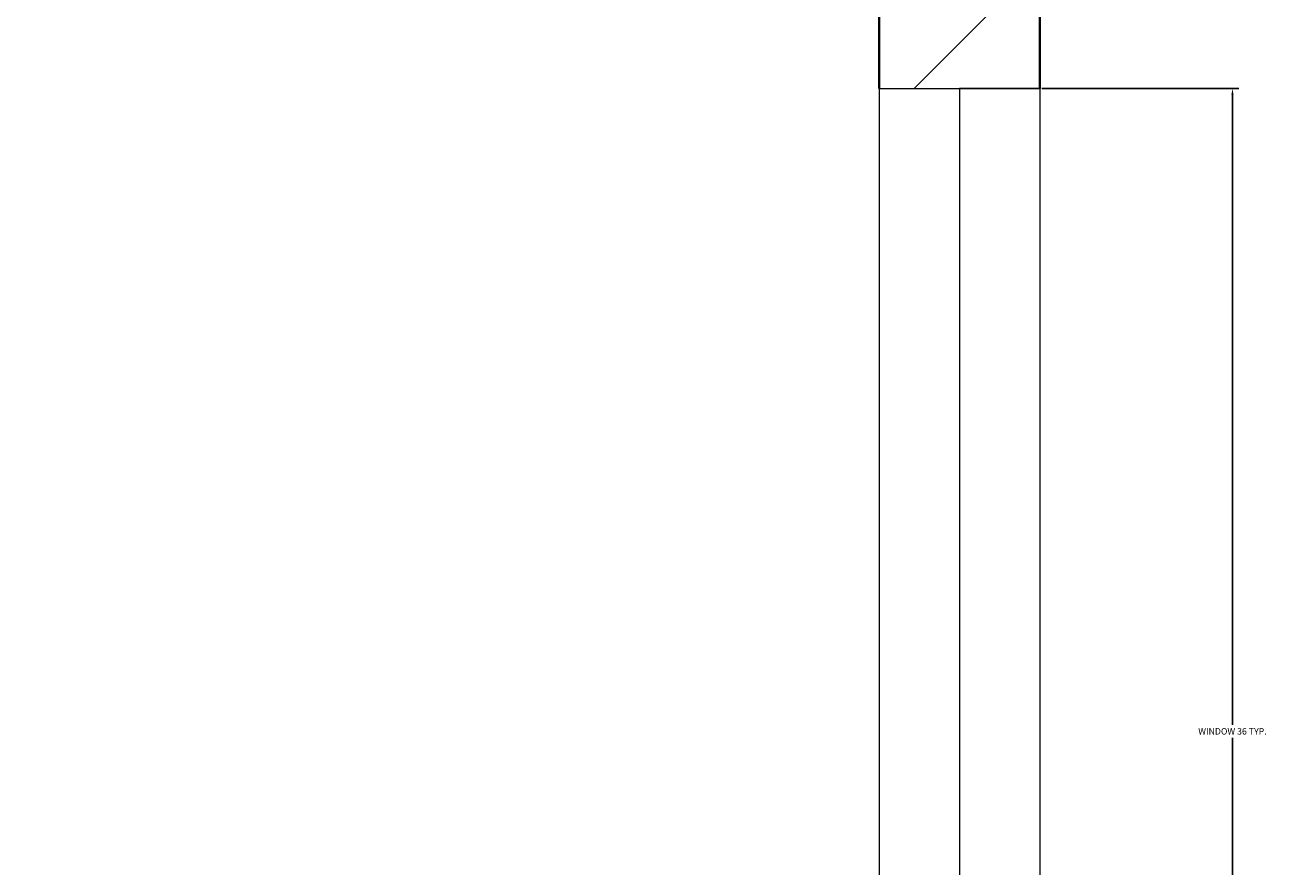
# Model space of a CAD drawing. Units: inches. Extents: x 1885 to 2748, y 783 to 2421.
# Tile 75 of 117: x 1969 to 2004, y 2120 to 2144. Entities that reach past the tile are written whole.
import ezdxf

# ---------------------------------------------------------------- set-up
doc = ezdxf.new("R2010")
doc.units = ezdxf.units.IN
for name, color, linetype, lineweight in [('A-ANNO-DIMS', 2, 'Continuous', 18), ('A-GLAZ', 181, 'Continuous', 18), ('A-WALL', 7, 'Continuous', 35)]:
    doc.layers.add(name, color=color, linetype=linetype, lineweight=lineweight)
doc.layers.add('A-WALL-PATT', color=85, linetype='Continuous', lineweight=13, true_color=0x58ba48)
doc.styles.get("Standard").update_dxf_attribs({"font": 'arial.ttf'})
doc.dimstyles.get("Standard").update_dxf_attribs({"dimtxt": 0.18, "dimasz": 0.18, "dimexe": 0.18, "dimexo": 0.0625, "dimgap": 0.09, "dimtad": 0, "dimtih": 1, "dimtoh": 1, "dimdec": 4, "dimzin": 0, "dimdsep": 46, "dimtxsty": 'Standard', "dimcen": 0.09, "dimadec": 0, "dimazin": 0, "dimtfac": 1, "dimtdec": 4, "dimtofl": 0, "dimtmove": 0, "dimatfit": 3, "dimfxl": 1, "dimtolj": 1, "dimtzin": 0, "dimarcsym": 0})

# ---------------------------------------------------------------- blocks, each defined once
blk = doc.blocks.new('WIN-36')
for p, q in [((0.004, 35.998), (4.504, 35.998)), ((0.004, 35.998), (0.004, -0.002)), ((4.504, 35.998), (2.254, 35.998)), ((2.254, 35.998), (2.254, -0.002)), ((4.504, 35.998), (4.504, -0.002)), ((2.254, -0.002), (0.004, -0.002)), ((0.004, -0.002), (4.504, -0.002))]:
    blk.add_line(p, q)
blk = doc.blocks.new('*D19')
at = {"layer": 'A-ANNO-DIMS', "color": 0, "lineweight": -2, "transparency": 16777216}
for p, q in [((1997.336, 2141.927), (2002.854, 2141.927)), ((2002.674, 2141.747), (2002.674, 2124.11)), ((2002.674, 2106.107), (2002.674, 2123.744)), ((1997.336, 2105.927), (2002.854, 2105.927))]:
    blk.add_line(p, q, dxfattribs=at)
at = {"layer": 'A-ANNO-DIMS', "color": 0, "transparency": 16777216}
for points in [[(2002.644, 2141.747), (2002.704, 2141.747), (2002.674, 2141.927)], [(2002.644, 2106.107), (2002.704, 2106.107), (2002.674, 2105.927)]]:
    blk.add_solid(points, dxfattribs=at)
at = {"layer": 'Defpoints', "color": 0, "transparency": 16777216}
for p in [(1997.274, 2141.927), (2002.674, 2141.927), (1997.274, 2105.927)]:
    blk.add_point(p, dxfattribs=at)
at = {"layer": 'A-ANNO-DIMS', "color": 0, "transparency": 16777216, "insert": (2002.674, 2123.927), "char_height": 0.18, "attachment_point": 5}
blk.add_mtext('\\A1;WINDOW 36 TYP.', dxfattribs=at)
blk = doc.blocks.new('*D48')
at = {"layer": 'A-ANNO-DIMS', "color": 0, "lineweight": -2, "transparency": 16777216}
for p, q in [((1980.711, 2348.006), (1902.844, 2348.006)), ((1903.024, 2347.826), (1903.024, 2114.937)), ((1903.024, 1881.686), (1903.024, 2114.574)), ((2016.711, 1881.506), (1902.844, 1881.506))]:
    blk.add_line(p, q, dxfattribs=at)
at = {"layer": 'A-ANNO-DIMS', "color": 0, "transparency": 16777216}
for points in [[(1902.994, 2347.826), (1903.054, 2347.826), (1903.024, 2348.006)], [(1902.994, 1881.686), (1903.054, 1881.686), (1903.024, 1881.506)]]:
    blk.add_solid(points, dxfattribs=at)
at = {"layer": 'Defpoints', "color": 0, "transparency": 16777216}
for p in [(1903.024, 2348.006), (1980.774, 2348.006), (2016.774, 1881.506)]:
    blk.add_point(p, dxfattribs=at)
at = {"layer": 'A-ANNO-DIMS', "color": 0, "transparency": 16777216, "insert": (1903.024, 2114.756), "char_height": 0.18, "attachment_point": 5}
blk.add_mtext('\\A1;466.5', dxfattribs=at)

msp = doc.modelspace()

# ---------------------------------------------------------------- hatches: boundary and pattern name
at = {"layer": 'A-WALL-PATT'}
h = msp.add_hatch(dxfattribs=at)
h.set_pattern_fill('ANSI32', color=256)
h.paths.add_polyline_path([(2007.772, 2318.006), (1980.774, 2318.006), (1980.774, 2281.215), (1985.274, 2281.215), (1985.274, 2313.506), (2007.772, 2313.506), (2007.772, 2315.756)])
h.paths.add_polyline_path([(2094.324, 2318.006), (2067.772, 2318.006), (2067.772, 2313.506), (2094.324, 2313.506), (2094.324, 2315.756)])
h.paths.add_polyline_path([(2131.367, 2315.756), (2131.367, 2318.006), (2131.189, 2318.006), (2112.609, 2318.006), (2112.609, 2313.506), (2117.274, 2313.506), (2117.274, 2255.201), (2121.774, 2255.201), (2121.774, 2313.506), (2131.367, 2313.506)])
h.paths.add_polyline_path([(2190.512, 2318.006), (2155.367, 2318.006), (2155.367, 2313.506), (2169.774, 2313.506), (2169.774, 2229.506), (2121.774, 2229.506), (2121.774, 2233.451), (2119.524, 2233.451), (2117.274, 2233.451), (2117.274, 2201.101), (2121.774, 2201.101), (2121.774, 2225.006), (2169.774, 2225.006), (2169.774, 2165.006), (2306.274, 2165.006), (2306.274, 2066.006), (2310.774, 2066.006), (2344.274, 2066.006), (2486.274, 2066.006), (2486.274, 1886.006), (2483.02, 1886.006), (2483.02, 1881.506), (2486.274, 1881.506), (2486.274, 1880.678), (2490.774, 1880.678), (2490.774, 2070.506), (2344.274, 2070.506), (2310.774, 2070.506), (2310.774, 2165.006), (2310.774, 2173.636), (2308.524, 2173.636), (2306.274, 2173.636), (2306.274, 2169.506), (2174.274, 2169.506), (2174.274, 2313.506), (2190.512, 2313.506), (2190.512, 2315.756)])
h.paths.add_polyline_path([(1985.274, 2221.215), (1980.774, 2221.215), (1980.774, 2165.006), (1992.774, 2165.006), (1992.774, 2141.927), (1997.274, 2141.927), (1997.274, 2165.006), (2117.274, 2165.006), (2117.274, 2163.126), (2121.774, 2163.126), (2121.774, 2172.734), (2119.524, 2172.734), (2117.274, 2172.734), (2117.274, 2169.506), (1985.274, 2169.506)])
h.paths.add_polyline_path([(1997.274, 2105.927), (1992.774, 2105.927), (1992.774, 2070.506), (2016.774, 2070.506), (2016.774, 2059.123), (2019.024, 2059.123), (2021.274, 2059.123), (2021.274, 2070.506), (2117.274, 2070.506), (2117.274, 2022.506), (2114.423, 2022.506), (2114.423, 2018.006), (2123.627, 2018.006), (2123.627, 2020.256), (2123.627, 2022.506), (2121.774, 2022.506), (2121.774, 2142.587), (2119.524, 2142.587), (2117.274, 2142.587), (2117.274, 2075.006), (1997.274, 2075.006)])
h.paths.add_polyline_path([(2092.029, 2020.256), (2092.029, 2022.506), (2021.274, 2022.506), (2021.274, 2035.123), (2016.774, 2035.123), (2016.774, 2018.006), (2016.774, 1978.784), (2021.274, 1978.784), (2021.274, 2018.006), (2092.029, 2018.006)])
h.paths.add_polyline_path([(2260.938, 2022.506), (2153.105, 2022.506), (2153.105, 2020.256), (2153.105, 2018.006), (2155.274, 2018.006), (2155.274, 1886.006), (2107.629, 1886.006), (2107.629, 1881.506), (2182.911, 1881.506), (2182.911, 1883.756), (2182.911, 1886.006), (2159.774, 1886.006), (2159.774, 2018.006), (2260.938, 2018.006), (2260.938, 2020.256)])
h.paths.add_polyline_path([(2047.629, 1883.756), (2047.629, 1886.006), (2021.274, 1886.006), (2021.274, 1918.784), (2019.024, 1918.784), (2016.774, 1918.784), (2016.774, 1881.506), (2047.629, 1881.506)])
h.paths.add_polyline_path([(2306.361, 1883.756), (2306.361, 1886.006), (2296.274, 1886.006), (2296.274, 1982.006), (2316.535, 1982.006), (2316.535, 1984.256), (2316.535, 1986.506), (2296.274, 1986.506), (2296.274, 2022.506), (2289.276, 2022.506), (2289.276, 2018.006), (2291.774, 2018.006), (2291.774, 1886.006), (2242.911, 1886.006), (2242.911, 1881.506), (2306.361, 1881.506)], flags=17)
h.paths.add_polyline_path([(1985.274, 1843.006), (2021.6, 1843.006), (2021.534, 1845.441), (2021.477, 1847.506), (1980.774, 1847.506), (1980.774, 1809.446), (1985.274, 1809.446)])
h.paths.add_polyline_path([(2131.482, 1845.256), (2131.482, 1847.506), (2081.534, 1847.506), (2081.534, 1843.006), (2117.274, 1843.006), (2117.274, 1784.147), (2119.524, 1784.147), (2121.774, 1784.147), (2121.774, 1843.006), (2131.482, 1843.006)])
h.paths.add_polyline_path([(2203.886, 1847.506), (2155.482, 1847.506), (2155.482, 1843.006), (2169.774, 1843.006), (2169.774, 1759.006), (2121.774, 1759.006), (2121.774, 1761.457), (2117.274, 1761.457), (2117.274, 1730.429), (2121.774, 1730.429), (2121.774, 1754.506), (2177.421, 1754.506), (2177.421, 1756.756), (2177.421, 1759.006), (2174.274, 1759.006), (2174.274, 1843.006), (2203.886, 1843.006)])
h.paths.add_polyline_path([(2335.554, 1845.256), (2335.554, 1847.506), (2239.886, 1847.506), (2239.886, 1843.006), (2306.274, 1843.006), (2306.274, 1759.006), (2199.486, 1759.006), (2199.486, 1754.506), (2310.774, 1754.506), (2310.774, 1843.006), (2335.554, 1843.006)])
h.paths.add_polyline_path([(2348.774, 2022.506), (2344.274, 2022.506), (2344.274, 1986.506), (2341.681, 1986.506), (2341.681, 1982.006), (2344.274, 1982.006), (2344.274, 1886.006), (2330.361, 1886.006), (2330.361, 1881.506), (2361.627, 1881.506), (2361.627, 1883.756), (2361.627, 1886.006), (2348.774, 1886.006)], flags=17)
h.paths.add_polyline_path([(2283.251, 2315.756), (2283.251, 2318.006), (2238.512, 2318.006), (2238.512, 2313.506), (2283.251, 2313.506)], flags=17)
h.paths.add_polyline_path([(2363.274, 2348.006), (2388.677, 2348.006), (2388.677, 2350.256), (2388.677, 2352.506), (2358.774, 2352.506), (2358.774, 2348.006), (2358.774, 2318.006), (2344.481, 2318.006), (2344.481, 2313.506), (2358.774, 2313.506), (2358.774, 2229.506), (2310.774, 2229.506), (2310.774, 2231.952), (2306.274, 2231.952), (2306.274, 2205.611), (2310.774, 2205.611), (2310.774, 2225.006), (2358.774, 2225.006), (2358.774, 2211.506), (2452.329, 2211.506), (2452.329, 2213.756), (2452.329, 2216.006), (2363.274, 2216.006), (2363.274, 2318.006)])
h.paths.add_polyline_path([(2310.774, 2313.506), (2320.481, 2313.506), (2320.481, 2315.756), (2320.481, 2318.006), (2302.728, 2318.006), (2302.728, 2313.506), (2306.274, 2313.506), (2306.274, 2251.076), (2310.774, 2251.076)], flags=17)
h.paths.add_polyline_path([(2490.774, 2352.506), (2486.274, 2352.506), (2448.677, 2352.506), (2448.677, 2348.006), (2486.274, 2348.006), (2486.274, 2318.006), (2486.274, 2216.006), (2481.78, 2216.006), (2481.78, 2211.506), (2486.274, 2211.506), (2486.274, 2165.006), (2493.289, 2165.006), (2493.289, 2167.256), (2493.289, 2169.506), (2490.774, 2169.506), (2490.774, 2313.506), (2494.429, 2313.506), (2494.429, 2318.006), (2490.774, 2318.006)])
h.paths.add_polyline_path([(2534.653, 2318.006), (2515.691, 2318.006), (2515.691, 2313.506), (2534.653, 2313.506), (2534.653, 2315.756)])
h.paths.add_polyline_path([(2618.274, 2318.006), (2594.653, 2318.006), (2594.653, 2313.506), (2613.774, 2313.506), (2613.774, 2281.706), (2618.274, 2281.706)])
h.paths.add_polyline_path([(2618.274, 2221.706), (2613.774, 2221.706), (2613.774, 2169.506), (2554.019, 2169.506), (2554.019, 2165.006), (2613.774, 2165.006), (2613.774, 2152.878), (2618.274, 2152.878)])
h.paths.add_polyline_path([(2618.274, 2128.878), (2616.024, 2128.878), (2613.774, 2128.878), (2613.774, 2117.006), (2529.774, 2117.006), (2529.774, 2165.006), (2532.848, 2165.006), (2532.848, 2169.506), (2522.867, 2169.506), (2522.867, 2165.006), (2525.274, 2165.006), (2525.274, 2117.006), (2525.274, 2112.506), (2525.274, 2108.576), (2529.774, 2108.576), (2529.774, 2112.506), (2613.774, 2112.506), (2613.774, 2080.19), (2618.274, 2080.19)])
h.paths.add_polyline_path([(2618.274, 2044.19), (2616.024, 2044.19), (2613.774, 2044.19), (2613.774, 2015.506), (2529.774, 2015.506), (2529.774, 2088.582), (2527.524, 2088.582), (2525.274, 2088.582), (2525.274, 2011.006), (2613.774, 2011.006), (2613.774, 1956.755), (2618.274, 1956.755)])
h.paths.add_polyline_path([(2618.274, 1881.506), (2618.274, 1896.755), (2613.774, 1896.755), (2613.774, 1881.506), (2613.774, 1847.506), (2592.715, 1847.506), (2592.715, 1843.006), (2613.774, 1843.006), (2613.774, 1765.006), (2613.774, 1760.506), (2609.621, 1760.506), (2609.621, 1756.006), (2613.774, 1756.006), (2613.774, 1660.006), (2608.544, 1660.006), (2608.544, 1655.506), (2613.774, 1655.506), (2613.774, 1508.158), (2618.274, 1508.158)])
h.paths.add_polyline_path([(2565.774, 1843.006), (2568.997, 1843.006), (2568.997, 1847.506), (2490.774, 1847.506), (2490.774, 1849.7), (2488.524, 1849.7), (2486.274, 1849.7), (2486.274, 1847.506), (2477.274, 1847.506), (2477.274, 1838.506), (2477.274, 1821.493), (2486.274, 1821.493), (2486.274, 1838.506), (2561.274, 1838.506), (2561.274, 1765.006), (2486.274, 1765.006), (2486.274, 1786.157), (2477.274, 1786.157), (2477.274, 1765.006), (2477.274, 1756.006), (2486.274, 1756.006), (2565.774, 1756.006), (2585.621, 1756.006), (2585.621, 1758.256), (2585.621, 1760.506), (2565.774, 1760.506), (2565.774, 1765.006)])
h.paths.add_polyline_path([(2486.274, 1651.006), (2561.274, 1651.006), (2561.274, 1567.006), (2486.274, 1567.006), (2486.274, 1591.321), (2477.274, 1591.321), (2477.274, 1567.006), (2477.274, 1558.006), (2477.274, 1555.439), (2481.774, 1555.439), (2481.774, 1558.006), (2568.653, 1558.006), (2568.653, 1560.256), (2568.653, 1562.506), (2565.774, 1562.506), (2565.774, 1655.506), (2584.544, 1655.506), (2584.544, 1657.756), (2584.544, 1660.006), (2565.774, 1660.006), (2486.274, 1660.006), (2477.274, 1660.006), (2477.274, 1651.006), (2477.274, 1632.989), (2486.274, 1632.989)])
h.paths.add_polyline_path([(2449.967, 1883.756), (2449.967, 1886.006), (2421.627, 1886.006), (2421.627, 1881.506), (2449.967, 1881.506)], flags=17)
h.paths.add_polyline_path([(2447.274, 1847.506), (2395.554, 1847.506), (2395.554, 1843.006), (2442.774, 1843.006), (2442.774, 1809.27), (2447.274, 1809.27)])
h.paths.add_polyline_path([(1985.274, 1749.446), (1980.774, 1749.446), (1980.774, 1694.504), (1985.274, 1694.504), (1985.274, 1694.506), (1986.897, 1694.506), (1986.897, 1697.78), (1986.897, 1699.006), (1985.274, 1699.006)])
h.paths.add_polyline_path([(2152.774, 1699.006), (2121.774, 1699.006), (2121.774, 1703.668), (2119.524, 1703.668), (2117.274, 1703.668), (2117.274, 1699.006), (2009.219, 1699.006), (2009.219, 1694.506), (2148.274, 1694.506), (2148.274, 1692.631), (2152.774, 1692.631)])
h.paths.add_polyline_path([(2016.274, 1694.506), (2011.774, 1694.506), (2011.774, 1558.006), (2040.806, 1558.006), (2040.806, 1560.256), (2040.806, 1562.506), (2016.274, 1562.506)])
h.paths.add_polyline_path([(2152.774, 1663.017), (2150.524, 1663.017), (2148.274, 1663.017), (2148.274, 1562.506), (2100.806, 1562.506), (2100.806, 1558.006), (2165.119, 1558.006), (2165.119, 1560.256), (2165.119, 1562.506), (2152.774, 1562.506), (2152.774, 1610.506), (2224.774, 1610.506), (2224.774, 1607.99), (2229.274, 1607.99), (2229.274, 1615.006), (2152.774, 1615.006)])
h.paths.add_polyline_path([(2238.613, 1560.256), (2238.613, 1562.506), (2229.274, 1562.506), (2229.274, 1588.756), (2227.024, 1588.763), (2224.774, 1588.771), (2224.774, 1562.506), (2189.119, 1562.506), (2189.119, 1558.006), (2238.613, 1558.006)])
h.paths.add_polyline_path([(2336.024, 1560.256), (2336.024, 1562.506), (2310.774, 1562.506), (2310.774, 1656.347), (2308.524, 1656.347), (2306.274, 1656.347), (2306.274, 1562.506), (2286.613, 1562.506), (2286.613, 1558.006), (2336.024, 1558.006)])
h.paths.add_polyline_path([(2447.274, 1690.968), (2445.024, 1690.968), (2442.774, 1690.968), (2442.774, 1687.006), (2306.274, 1687.006), (2306.274, 1680.75), (2310.774, 1680.75), (2310.774, 1682.506), (2442.774, 1682.506), (2442.774, 1562.506), (2396.024, 1562.506), (2396.024, 1558.006), (2447.274, 1558.006)])
h.paths.add_polyline_path([(2447.274, 1749.27), (2445.024, 1749.27), (2442.774, 1749.27), (2442.774, 1717.232), (2447.274, 1717.232)])
h.paths.add_polyline_path([(2044.674, 1521.756), (2044.674, 1524.006), (2007.274, 1524.006), (2007.274, 1503.49), (2009.524, 1503.49), (2011.774, 1503.49), (2011.774, 1519.506), (2044.674, 1519.506)])
h.paths.add_polyline_path([(2177.969, 1521.756), (2177.969, 1524.006), (2104.674, 1524.006), (2104.674, 1519.506), (2145.774, 1519.506), (2145.774, 1387.506), (2143.37, 1387.506), (2143.37, 1383.006), (2251.585, 1383.006), (2251.585, 1385.256), (2251.585, 1387.506), (2150.274, 1387.506), (2150.274, 1519.506), (2177.969, 1519.506)])
h.paths.add_polyline_path([(2298.704, 1524.006), (2237.969, 1524.006), (2237.969, 1519.506), (2282.274, 1519.506), (2282.274, 1387.506), (2279.683, 1387.506), (2279.683, 1383.006), (2286.774, 1383.006), (2286.774, 1419.006), (2312.451, 1419.006), (2312.451, 1421.256), (2312.451, 1423.506), (2286.774, 1423.506), (2286.774, 1519.506), (2298.704, 1519.506), (2298.704, 1521.722)], flags=17)
h.paths.add_polyline_path([(2361.897, 1521.756), (2361.897, 1524.006), (2322.704, 1524.006), (2322.704, 1519.506), (2334.774, 1519.506), (2334.774, 1423.506), (2331.93, 1423.506), (2331.93, 1419.006), (2334.774, 1419.006), (2334.774, 1387.506), (2334.774, 1383.228), (2339.274, 1383.228), (2339.274, 1387.506), (2339.274, 1519.506), (2361.897, 1519.506)], flags=17)
h.paths.add_polyline_path([(2447.274, 1521.756), (2447.274, 1524.006), (2421.897, 1524.006), (2421.897, 1519.506), (2447.274, 1519.506)], flags=17)
h.paths.add_polyline_path([(2481.774, 1529.6), (2479.524, 1529.6), (2477.274, 1529.6), (2477.274, 1524.006), (2474.489, 1524.006), (2474.489, 1519.506), (2477.274, 1519.506), (2477.274, 1334.506), (2296.774, 1334.506), (2296.774, 1240.506), (2160.274, 1240.506), (2160.274, 1180.506), (2112.274, 1180.506), (2112.274, 1207.692), (2110.024, 1207.692), (2107.774, 1207.692), (2107.774, 1171.609), (2112.274, 1171.609), (2112.274, 1176.006), (2160.274, 1176.006), (2160.274, 1092.006), (2144.221, 1092.006), (2144.221, 1087.506), (2189.497, 1087.506), (2189.497, 1089.756), (2189.497, 1092.006), (2164.774, 1092.006), (2164.774, 1236.006), (2296.774, 1236.006), (2296.774, 1231.912), (2301.274, 1231.912), (2301.274, 1330.006), (2481.774, 1330.006), (2481.774, 1387.506)])
h.paths.add_polyline_path([(2618.274, 1448.158), (2613.774, 1448.158), (2613.774, 1382.506), (2529.774, 1382.506), (2525.274, 1382.506), (2525.274, 1307.062), (2529.774, 1307.062), (2529.774, 1378.006), (2613.774, 1378.006), (2613.774, 1354.988), (2618.274, 1354.988)])
h.paths.add_polyline_path([(2618.274, 1318.988), (2613.774, 1318.988), (2613.774, 1281.006), (2529.774, 1281.006), (2529.774, 1283.786), (2527.524, 1283.786), (2525.274, 1283.786), (2525.274, 1228.506), (2516.794, 1228.506), (2516.794, 1224.006), (2533.484, 1224.006), (2533.484, 1226.256), (2533.484, 1228.506), (2529.774, 1228.506), (2529.774, 1276.506), (2613.774, 1276.506), (2613.774, 1266.02), (2618.274, 1266.02)])
h.paths.add_polyline_path([(2618.274, 1134.964), (2613.774, 1134.964), (2613.774, 1092.006), (2594.545, 1092.006), (2594.545, 1087.506), (2618.274, 1087.506)])
h.paths.add_polyline_path([(2534.545, 1092.006), (2509.765, 1092.006), (2509.765, 1087.506), (2534.545, 1087.506), (2534.545, 1089.756)])
h.paths.add_polyline_path([(2481.274, 1224.006), (2484.117, 1224.006), (2484.117, 1226.256), (2484.117, 1228.506), (2476.774, 1228.506), (2476.774, 1198.506), (2471.61, 1198.506), (2471.61, 1194.006), (2476.774, 1194.006), (2476.774, 1062.006), (2436.894, 1062.006), (2436.894, 1057.506), (2476.774, 1057.506), (2481.274, 1057.506), (2481.274, 1062.006), (2481.274, 1087.506), (2485.354, 1087.506), (2485.354, 1089.756), (2485.354, 1092.006), (2481.274, 1092.006), (2481.274, 1117.506)])
h.paths.add_polyline_path([(2439.898, 1198.506), (2349.274, 1198.506), (2349.274, 1194.006), (2349.274, 1180.506), (2301.274, 1180.506), (2301.274, 1201.896), (2299.024, 1201.896), (2296.774, 1201.896), (2296.774, 1172.335), (2299.024, 1172.335), (2301.274, 1172.335), (2301.274, 1176.006), (2349.274, 1176.006), (2349.274, 1092.006), (2334.452, 1092.006), (2334.452, 1087.506), (2349.274, 1087.506), (2349.274, 1057.506), (2353.774, 1057.506), (2376.894, 1057.506), (2376.894, 1059.756), (2376.894, 1062.006), (2353.774, 1062.006), (2353.774, 1087.506), (2353.774, 1180.506), (2353.774, 1194.006), (2439.898, 1194.006), (2439.898, 1196.256)])
h.paths.add_polyline_path([(2270.596, 1089.756), (2270.596, 1092.006), (2249.497, 1092.006), (2249.497, 1087.506), (2270.596, 1087.506)], flags=17)
h.paths.add_polyline_path([(2310.452, 1092.006), (2301.274, 1092.006), (2301.274, 1153.292), (2296.774, 1153.292), (2296.774, 1092.006), (2293.786, 1092.006), (2293.786, 1087.506), (2310.452, 1087.506), (2310.452, 1089.756)], flags=17)
h.paths.add_polyline_path([(2112.274, 1150.328), (2110.024, 1150.328), (2107.774, 1150.328), (2107.774, 1092.006), (2104.465, 1092.006), (2104.465, 1087.506), (2120.221, 1087.506), (2120.221, 1089.756), (2120.221, 1092.006), (2112.274, 1092.006)])
h.paths.add_polyline_path([(2082.172, 1092.006), (2058.144, 1092.006), (2058.144, 1087.506), (2082.172, 1087.506), (2082.172, 1089.756)])
h.paths.add_polyline_path([(1975.774, 1145.638), (1971.274, 1145.638), (1971.274, 1087.506), (1980.774, 1087.506), (1998.144, 1087.506), (1998.144, 1089.756), (1998.144, 1092.006), (1985.274, 1092.006), (1975.774, 1092.006)])
h.paths.add_polyline_path([(2112.274, 1244.385), (2110.024, 1244.385), (2107.774, 1244.385), (2107.774, 1240.506), (1992.274, 1240.506), (1992.274, 1271.008), (1987.774, 1271.008), (1987.774, 1240.506), (1980.774, 1240.506), (1975.774, 1240.506), (1971.274, 1240.506), (1971.274, 1205.638), (1975.774, 1205.638), (1975.774, 1236.006), (2107.774, 1236.006), (2107.774, 1233.444), (2112.274, 1233.444), (2112.274, 1236.006)])
h.paths.add_polyline_path([(2112.274, 1383.006), (2114.783, 1383.006), (2114.783, 1385.256), (2114.783, 1387.506), (2102.476, 1387.506), (2102.476, 1383.006), (2107.774, 1383.006), (2107.774, 1335.006), (2011.774, 1335.006), (2011.774, 1349.939), (2007.274, 1349.939), (2007.274, 1335.006), (1987.774, 1335.006), (1987.774, 1330.506), (1987.774, 1307.008), (1992.274, 1307.008), (1992.274, 1330.506), (2007.274, 1330.506), (2107.774, 1330.506), (2107.774, 1264.711), (2112.274, 1264.711)])
h.paths.add_polyline_path([(2077.857, 1387.506), (2011.774, 1387.506), (2011.774, 1390.036), (2009.524, 1390.036), (2007.274, 1390.036), (2007.274, 1373.939), (2011.774, 1373.939), (2011.774, 1383.006), (2077.857, 1383.006)])
h.paths.add_polyline_path([(2011.774, 1443.49), (2007.274, 1443.49), (2007.274, 1410.248), (2011.774, 1410.248)])

# ---------------------------------------------------------------- linework, layer by layer
at = {"layer": 'A-WALL'}
for p, q in [((1992.774, 2165.006), (1992.774, 2141.927)), ((1997.274, 2165.006), (1997.274, 2141.927))]:
    msp.add_line(p, q, dxfattribs=at)

# ---------------------------------------------------------------- block references
at = {"layer": 'A-GLAZ'}
msp.add_blockref('WIN-36', (1992.77, 2105.929), dxfattribs=at)

# ---------------------------------------------------------------- dimensions: what is measured, and where the dimension line sits
at = {"layer": 'A-ANNO-DIMS'}
dim = msp.add_linear_dim(base=(1903.024, 2348.006), p1=(2016.774, 1881.506), p2=(1980.774, 2348.006), angle=90, dimstyle='Standard', override={"dimdec": 1, "dimlfac": 1, "dimrnd": 0, "dimzin": 0, "dimdsep": 46, "dimlunit": 2}, dxfattribs=at)
dim.commit()
dim.dimension.update_dxf_attribs({"geometry": '*D48', "text_midpoint": (1903.024, 2114.756)})
dim = msp.add_linear_dim(base=(2002.674, 2141.927), p1=(1997.274, 2105.927), p2=(1997.274, 2141.927), angle=90, text='WINDOW <> TYP.', dimstyle='Standard', override={"dimdec": 0, "dimlfac": 1, "dimrnd": 0, "dimzin": 0, "dimdsep": 46, "dimlunit": 2}, dxfattribs=at)
dim.commit()
dim.dimension.update_dxf_attribs({"geometry": '*D19', "text_midpoint": (2002.674, 2123.927)})

doc.saveas('drawing.dxf')
